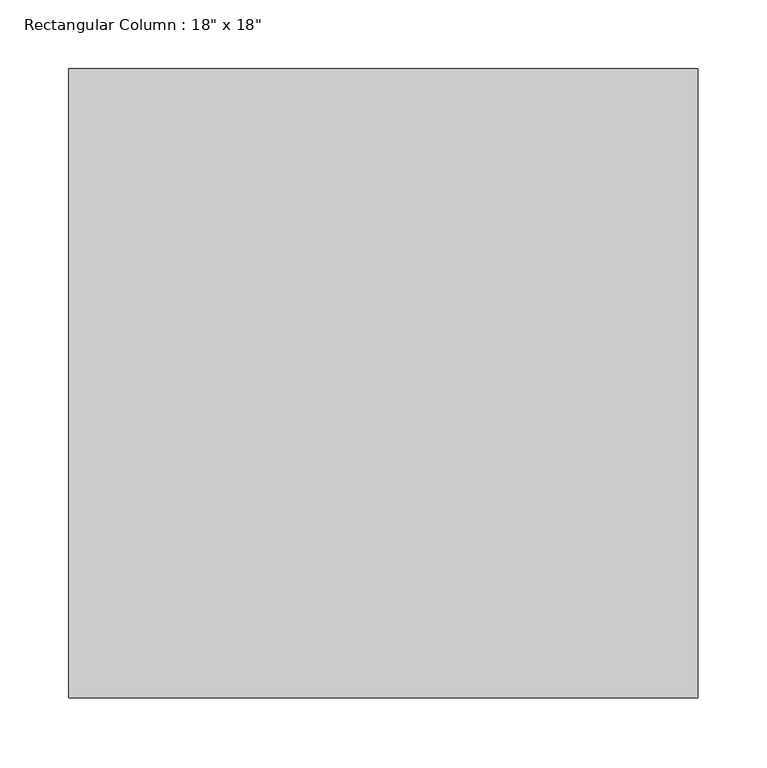
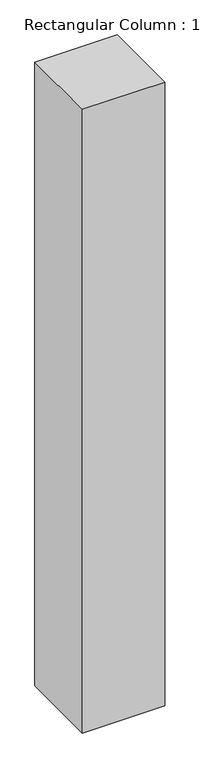
"""IFC4 building model written with IfcOpenShell, lengths in millimetres: column geometry."""

from ifc_helpers import new_model, si_unit, origin, origin_with_axes, place, context, project, spatial, polyline, outline, extrude, source, transform, mapped, element, save


def column_ce396696(model_context):
    return source(origin(), model_context, "Body", "SweptSolid", [
        extrude(outline(polyline([(228.6, 228.6), (228.6, -228.6), (-228.6, -228.6), (-228.6, 228.6), (228.6, 228.6)])), origin_with_axes(), (0.0, 0.0, 1.0), 3657.6),
    ])


if __name__ == "__main__":
    model = new_model("IFC4")
    model_context = context("Model", 3, world=origin())
    ifc_project = project(units=[si_unit("LENGTHUNIT", "METRE", prefix="MILLI")], contexts=[model_context])
    site = spatial("IfcSite", under=ifc_project)
    building = spatial("IfcBuilding", under=site)
    placement = place(None, origin())
    column_shape = column_ce396696(model_context)
    element("IfcColumn", 1, ObjectType="Rectangular Column : 18\" x 18\"", at=placement, inside=building, context=model_context, shape_type="MappedRepresentation", body=[
        mapped(column_shape, transform((0.0, 0.0, 0.0), x_axis=(1.0, 0.0, 0.0), y_axis=(0.0, 1.0, 0.0), z_axis=(0.0, 0.0, 1.0))),
    ])
    save(model, "model.ifc")

# Revit data of these elements
# Type "Rectangular Column : 18\" x 18\""
#   Assembly Code = "B1010200"
#   Depth = 1' - 6"
#   Offset Base = 0' - 0"
#   Offset Top = 0' - 0"
#   Width = 1' - 6"
#   Material = none
